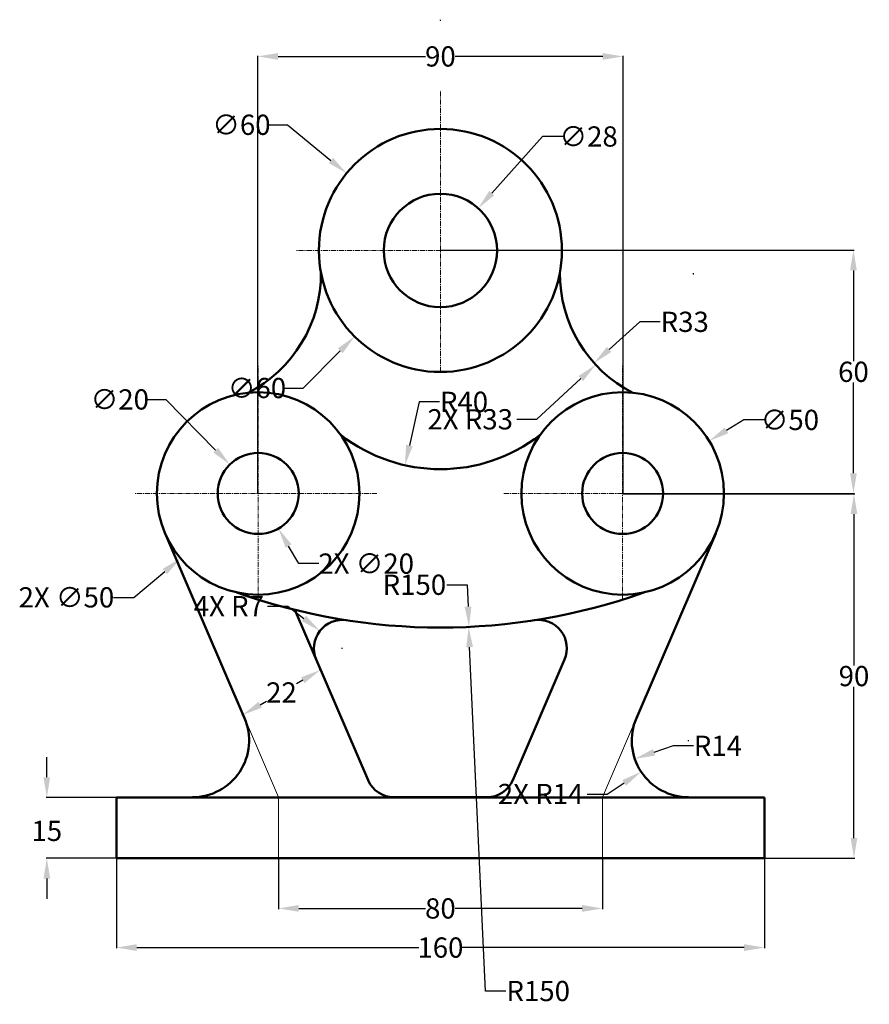
# Model space of a CAD drawing. Units: millimetres. Extents: x 106 to 316, y 45 to 288.
import ezdxf

# ---------------------------------------------------------------- set-up
doc = ezdxf.new("R2010")
doc.units = ezdxf.units.MM
doc.header["$MEASUREMENT"] = 0
doc.linetypes.add('CENTER', pattern=[2, 1.25, -0.25, 0.25, -0.25])
for name, color, linetype, lineweight in [('CENTER', 7, 'CENTER', 18), ('M-CONS', 8, 'Continuous', 13), ('M-DIMS', 2, 'Continuous', 25), ('M-OUTL', 7, 'Continuous', 50)]:
    doc.layers.add(name, color=color, linetype=linetype, lineweight=lineweight)
doc.styles.get("Standard").update_dxf_attribs({"font": 'arial.ttf'})
doc.dimstyles.get("Standard").update_dxf_attribs({"dimtxt": 5, "dimasz": 5, "dimexe": 0.18, "dimexo": 0.0625, "dimgap": 0.09, "dimtad": 0, "dimtih": 1, "dimtoh": 1, "dimdec": 0, "dimzin": 0, "dimdsep": 46, "dimtxsty": 'Standard', "dimcen": 0.09, "dimadec": 0, "dimazin": 0, "dimtfac": 1, "dimtdec": 0, "dimtofl": 0, "dimtmove": 0, "dimatfit": 3, "dimfxl": 1, "dimtolj": 1, "dimtzin": 0, "dimarcsym": 0})

# ---------------------------------------------------------------- blocks, each defined once
blk = doc.blocks.new('*D1')
at = {"layer": 'Defpoints', "color": 0, "transparency": 16777216}
for p in [(210.19, 217.04), (201.44, 178.01)]:
    blk.add_point(p, dxfattribs=at)
at = {"layer": 'M-DIMS', "color": 0, "lineweight": -2, "transparency": 16777216}
for p, q in [((204.95, 193.67), (202.53, 182.89)), ((209.95, 193.67), (204.95, 193.67))]:
    blk.add_line(p, q, dxfattribs=at)
at = {"layer": 'M-DIMS', "color": 0, "transparency": 16777216}
blk.add_solid([(201.72, 183.07), (203.35, 182.7), (201.44, 178.01)], dxfattribs=at)
at = {"layer": 'M-DIMS', "color": 0, "transparency": 16777216, "insert": (216.01, 193.67), "char_height": 5, "attachment_point": 5}
blk.add_mtext('\\A1;R40', dxfattribs=at)
blk = doc.blocks.new('*D2')
at = {"layer": 'Defpoints', "color": 0, "transparency": 16777216}
for p in [(210.19, 287.93), (217.25, 138.1)]:
    blk.add_point(p, dxfattribs=at)
at = {"layer": 'M-DIMS', "color": 0, "lineweight": -2, "transparency": 16777216}
for p, q in [((211.76, 148.5), (216.76, 148.5)), ((216.76, 148.5), (217.01, 143.09))]:
    blk.add_line(p, q, dxfattribs=at)
at = {"layer": 'M-DIMS', "color": 0, "transparency": 16777216}
blk.add_solid([(217.84, 143.13), (216.18, 143.05), (217.25, 138.1)], dxfattribs=at)
at = {"layer": 'M-DIMS', "color": 0, "transparency": 16777216, "insert": (203.76, 148.5), "char_height": 5, "attachment_point": 5}
blk.add_mtext('\\A1;R150', dxfattribs=at)
blk = doc.blocks.new('*D3')
at = {"layer": 'Defpoints', "color": 0, "transparency": 16777216}
for p in [(271.44, 110.04), (258.2, 105.5)]:
    blk.add_point(p, dxfattribs=at)
at = {"layer": 'M-DIMS', "color": 0, "lineweight": -2, "transparency": 16777216}
for p, q in [((267.66, 108.74), (262.93, 107.12)), ((272.66, 108.74), (267.66, 108.74))]:
    blk.add_line(p, q, dxfattribs=at)
at = {"layer": 'M-DIMS', "color": 0, "transparency": 16777216}
blk.add_solid([(262.66, 107.91), (263.2, 106.33), (258.2, 105.5)], dxfattribs=at)
at = {"layer": 'M-DIMS', "color": 0, "transparency": 16777216, "insert": (278.71, 108.74), "char_height": 5, "attachment_point": 5}
blk.add_mtext('\\A1;R14', dxfattribs=at)
blk = doc.blocks.new('*D4')
at = {"layer": 'Defpoints', "color": 0, "transparency": 16777216}
for p in [(272.69, 225.31), (248.14, 203.26)]:
    blk.add_point(p, dxfattribs=at)
at = {"layer": 'M-DIMS', "color": 0, "lineweight": -2, "transparency": 16777216}
for p, q in [((259.45, 213.42), (251.86, 206.6)), ((264.45, 213.42), (259.45, 213.42))]:
    blk.add_line(p, q, dxfattribs=at)
at = {"layer": 'M-DIMS', "color": 0, "transparency": 16777216}
blk.add_solid([(251.3, 207.22), (252.41, 205.98), (248.14, 203.26)], dxfattribs=at)
at = {"layer": 'M-DIMS', "color": 0, "transparency": 16777216, "insert": (270.52, 213.42), "char_height": 5, "attachment_point": 5}
blk.add_mtext('\\A1;R33', dxfattribs=at)
blk = doc.blocks.new('*D5')
at = {"layer": 'Defpoints', "color": 0, "transparency": 16777216}
for p in [(187.02, 250.09), (233.37, 211.99)]:
    blk.add_point(p, dxfattribs=at)
at = {"layer": 'M-DIMS', "color": 0, "lineweight": -2, "transparency": 16777216}
for p, q in [((167.43, 262.07), (172.43, 262.07)), ((172.43, 262.07), (183.15, 253.26)), ((210.1, 231.04), (210.28, 231.04)), ((210.19, 230.95), (210.19, 231.13))]:
    blk.add_line(p, q, dxfattribs=at)
at = {"layer": 'M-DIMS', "color": 0, "transparency": 16777216}
blk.add_solid([(183.68, 253.9), (182.63, 252.62), (187.02, 250.09)], dxfattribs=at)
at = {"layer": 'M-DIMS', "color": 0, "transparency": 16777216, "insert": (161.05, 262.07), "char_height": 5, "attachment_point": 5}
blk.add_mtext('\\A1;∅60', dxfattribs=at)
blk = doc.blocks.new('*D6')
at = {"layer": 'Defpoints', "color": 0, "transparency": 16777216}
for p in [(219.53, 241.47), (200.85, 220.61)]:
    blk.add_point(p, dxfattribs=at)
at = {"layer": 'M-DIMS', "color": 0, "lineweight": -2, "transparency": 16777216}
for p, q in [((235.39, 259.18), (222.87, 245.19)), ((240.39, 259.18), (235.39, 259.18)), ((210.1, 231.04), (210.28, 231.04)), ((210.19, 230.95), (210.19, 231.13))]:
    blk.add_line(p, q, dxfattribs=at)
at = {"layer": 'M-DIMS', "color": 0, "transparency": 16777216}
blk.add_solid([(222.25, 245.75), (223.49, 244.64), (219.53, 241.47)], dxfattribs=at)
at = {"layer": 'M-DIMS', "color": 0, "transparency": 16777216, "insert": (246.79, 259.18), "char_height": 5, "attachment_point": 5}
blk.add_mtext('\\A1;∅28', dxfattribs=at)
blk = doc.blocks.new('*D7')
at = {"layer": 'Defpoints', "color": 0, "transparency": 16777216}
for p in [(276.56, 184.01), (233.82, 158.06)]:
    blk.add_point(p, dxfattribs=at)
at = {"layer": 'M-DIMS', "color": 0, "lineweight": -2, "transparency": 16777216}
for p, q in [((285.11, 189.2), (280.84, 186.61)), ((290.11, 189.2), (285.11, 189.2)), ((255.1, 171.04), (255.28, 171.04)), ((255.19, 170.95), (255.19, 171.13))]:
    blk.add_line(p, q, dxfattribs=at)
at = {"layer": 'M-DIMS', "color": 0, "transparency": 16777216}
blk.add_solid([(280.41, 187.32), (281.27, 185.9), (276.56, 184.01)], dxfattribs=at)
at = {"layer": 'M-DIMS', "color": 0, "transparency": 16777216, "insert": (296.49, 189.2), "char_height": 5, "attachment_point": 5}
blk.add_mtext('\\A1;∅50', dxfattribs=at)
blk = doc.blocks.new('*D8')
at = {"layer": 'Defpoints', "color": 0, "transparency": 16777216}
for p in [(158.19, 178.18), (172.2, 163.9)]:
    blk.add_point(p, dxfattribs=at)
at = {"layer": 'M-DIMS', "color": 0, "lineweight": -2, "transparency": 16777216}
for p, q in [((137.4, 194.26), (142.4, 194.26)), ((142.4, 194.26), (154.69, 181.74)), ((165.1, 171.04), (165.28, 171.04)), ((165.19, 170.95), (165.19, 171.13))]:
    blk.add_line(p, q, dxfattribs=at)
at = {"layer": 'M-DIMS', "color": 0, "transparency": 16777216}
blk.add_solid([(155.28, 182.33), (154.09, 181.16), (158.19, 178.18)], dxfattribs=at)
at = {"layer": 'M-DIMS', "color": 0, "transparency": 16777216, "insert": (131.02, 194.26), "char_height": 5, "attachment_point": 5}
blk.add_mtext('\\A1;∅20', dxfattribs=at)
blk = doc.blocks.new('*D9')
at = {"layer": 'Defpoints', "color": 0, "transparency": 16777216}
for p in [(180.53, 127.44), (181, 126.64), (161.81, 115.56)]:
    blk.add_point(p, dxfattribs=at)
at = {"layer": 'M-DIMS', "color": 0, "lineweight": -2, "transparency": 16777216}
for p, q in [((180.96, 126.69), (180.44, 127.6)), ((176.2, 124.94), (174.63, 124.03)), ((165.68, 118.86), (167.25, 119.77)), ((161.78, 115.62), (161.26, 116.52))]:
    blk.add_line(p, q, dxfattribs=at)
at = {"layer": 'M-DIMS', "color": 0, "transparency": 16777216}
for points in [[(175.79, 125.66), (176.62, 124.22), (180.53, 127.44)], [(165.26, 119.58), (166.09, 118.14), (161.35, 116.36)]]:
    blk.add_solid(points, dxfattribs=at)
at = {"layer": 'M-DIMS', "color": 0, "transparency": 16777216, "insert": (170.94, 121.9), "char_height": 5, "attachment_point": 5}
blk.add_mtext('\\A1;22', dxfattribs=at)
blk = doc.blocks.new('*D10')
at = {"layer": 'Defpoints', "color": 0, "transparency": 16777216}
for p in [(255.28, 278.95), (165.1, 171.04), (255.28, 171.04)]:
    blk.add_point(p, dxfattribs=at)
at = {"layer": 'M-DIMS', "color": 0, "lineweight": -2, "transparency": 16777216}
for p, q in [((165.1, 171.1), (165.1, 279.13)), ((170.1, 278.95), (206.53, 278.95)), ((250.28, 278.95), (213.86, 278.95)), ((255.28, 171.1), (255.28, 279.13))]:
    blk.add_line(p, q, dxfattribs=at)
at = {"layer": 'M-DIMS', "color": 0, "transparency": 16777216}
for points in [[(170.1, 279.78), (170.1, 278.12), (165.1, 278.95)], [(250.28, 279.78), (250.28, 278.12), (255.28, 278.95)]]:
    blk.add_solid(points, dxfattribs=at)
at = {"layer": 'M-DIMS', "color": 0, "transparency": 16777216, "insert": (210.19, 278.95), "char_height": 5, "attachment_point": 5}
blk.add_mtext('\\A1;90', dxfattribs=at)
blk = doc.blocks.new('*D11')
at = {"layer": 'Defpoints', "color": 0, "transparency": 16777216}
for p in [(210.19, 231.13), (255.28, 171.04), (312.18, 171.04)]:
    blk.add_point(p, dxfattribs=at)
at = {"layer": 'M-DIMS', "color": 0, "lineweight": -2, "transparency": 16777216}
for p, q in [((210.26, 231.13), (312.36, 231.13)), ((312.18, 226.13), (312.18, 203.73)), ((312.18, 176.04), (312.18, 198.44)), ((255.35, 171.04), (312.36, 171.04))]:
    blk.add_line(p, q, dxfattribs=at)
at = {"layer": 'M-DIMS', "color": 0, "transparency": 16777216}
for points in [[(311.34, 226.13), (313.01, 226.13), (312.18, 231.13)], [(311.34, 176.04), (313.01, 176.04), (312.18, 171.04)]]:
    blk.add_solid(points, dxfattribs=at)
at = {"layer": 'M-DIMS', "color": 0, "transparency": 16777216, "insert": (312.18, 201.08), "char_height": 5, "attachment_point": 5}
blk.add_mtext('\\A1;60', dxfattribs=at)
blk = doc.blocks.new('*D12')
at = {"layer": 'Defpoints', "color": 0, "transparency": 16777216}
for p in [(255.19, 170.95), (255.19, 80.95), (312.31, 80.95)]:
    blk.add_point(p, dxfattribs=at)
at = {"layer": 'M-DIMS', "color": 0, "lineweight": -2, "transparency": 16777216}
for p, q in [((255.26, 170.95), (312.49, 170.95)), ((312.31, 165.95), (312.31, 128.59)), ((312.31, 85.95), (312.31, 123.31)), ((255.26, 80.95), (312.49, 80.95))]:
    blk.add_line(p, q, dxfattribs=at)
at = {"layer": 'M-DIMS', "color": 0, "transparency": 16777216}
for points in [[(311.48, 165.95), (313.14, 165.95), (312.31, 170.95)], [(311.48, 85.95), (313.14, 85.95), (312.31, 80.95)]]:
    blk.add_solid(points, dxfattribs=at)
at = {"layer": 'M-DIMS', "color": 0, "transparency": 16777216, "insert": (312.31, 125.95), "char_height": 5, "attachment_point": 5}
blk.add_mtext('\\A1;90', dxfattribs=at)
blk = doc.blocks.new('*D13')
at = {"layer": 'Defpoints', "color": 0, "transparency": 16777216}
for p in [(170.19, 80.95), (250.19, 80.95), (250.19, 68.58)]:
    blk.add_point(p, dxfattribs=at)
at = {"layer": 'M-DIMS', "color": 0, "lineweight": -2, "transparency": 16777216}
for p, q in [((170.19, 80.89), (170.19, 68.4)), ((250.19, 80.89), (250.19, 68.4)), ((175.19, 68.58), (206.53, 68.58)), ((245.19, 68.58), (213.86, 68.58))]:
    blk.add_line(p, q, dxfattribs=at)
at = {"layer": 'M-DIMS', "color": 0, "transparency": 16777216}
for points in [[(175.19, 69.42), (175.19, 67.75), (170.19, 68.58)], [(245.19, 69.42), (245.19, 67.75), (250.19, 68.58)]]:
    blk.add_solid(points, dxfattribs=at)
at = {"layer": 'M-DIMS', "color": 0, "transparency": 16777216, "insert": (210.19, 68.58), "char_height": 5, "attachment_point": 5}
blk.add_mtext('\\A1;80', dxfattribs=at)
blk = doc.blocks.new('*D14')
at = {"layer": 'Defpoints', "color": 0, "transparency": 16777216}
for p in [(130.19, 95.95), (113, 80.95), (130.19, 80.95)]:
    blk.add_point(p, dxfattribs=at)
at = {"layer": 'M-DIMS', "color": 0, "lineweight": -2, "transparency": 16777216}
for p, q in [((113, 100.95), (113, 105.95)), ((130.13, 95.95), (112.82, 95.95)), ((130.13, 80.95), (112.82, 80.95)), ((113, 75.95), (113, 70.95))]:
    blk.add_line(p, q, dxfattribs=at)
at = {"layer": 'M-DIMS', "color": 0, "transparency": 16777216}
for points in [[(112.17, 100.95), (113.83, 100.95), (113, 95.95)], [(112.17, 75.95), (113.83, 75.95), (113, 80.95)]]:
    blk.add_solid(points, dxfattribs=at)
at = {"layer": 'M-DIMS', "color": 0, "transparency": 16777216, "insert": (113, 87.73), "char_height": 5, "attachment_point": 5}
blk.add_mtext('\\A1;15', dxfattribs=at)
blk = doc.blocks.new('*D15')
at = {"layer": 'Defpoints', "color": 0, "transparency": 16777216}
for p in [(130.19, 80.95), (290.19, 80.95), (290.19, 58.92)]:
    blk.add_point(p, dxfattribs=at)
at = {"layer": 'M-DIMS', "color": 0, "lineweight": -2, "transparency": 16777216}
for p, q in [((130.19, 80.89), (130.19, 58.74)), ((290.19, 80.89), (290.19, 58.74)), ((135.19, 58.92), (204.82, 58.92)), ((285.19, 58.92), (215.56, 58.92))]:
    blk.add_line(p, q, dxfattribs=at)
at = {"layer": 'M-DIMS', "color": 0, "transparency": 16777216}
for points in [[(135.19, 59.75), (135.19, 58.08), (130.19, 58.92)], [(285.19, 59.75), (285.19, 58.08), (290.19, 58.92)]]:
    blk.add_solid(points, dxfattribs=at)
at = {"layer": 'M-DIMS', "color": 0, "transparency": 16777216, "insert": (210.19, 58.92), "char_height": 5, "attachment_point": 5}
blk.add_mtext('\\A1;160', dxfattribs=at)
blk = doc.blocks.new('BOSS-OD50-BORE20')
for radius in [25, 10]:
    blk.add_circle((25, 25), radius)
blk = doc.blocks.new('*D17')
at = {"layer": 'Defpoints', "color": 0, "transparency": 16777216}
for p in [(231.39, 252.27), (189, 209.81)]:
    blk.add_point(p, dxfattribs=at)
at = {"layer": 'M-DIMS', "color": 0, "lineweight": -2, "transparency": 16777216}
for p, q in [((210.1, 231.04), (210.28, 231.04)), ((210.19, 230.95), (210.19, 231.13)), ((176.28, 197.07), (185.47, 206.27)), ((171.28, 197.07), (176.28, 197.07))]:
    blk.add_line(p, q, dxfattribs=at)
at = {"layer": 'M-DIMS', "color": 0, "transparency": 16777216}
blk.add_solid([(184.88, 206.86), (186.06, 205.68), (189, 209.81)], dxfattribs=at)
at = {"layer": 'M-DIMS', "color": 0, "transparency": 16777216, "insert": (164.9, 197.07), "char_height": 5, "attachment_point": 5}
blk.add_mtext('\\A1;∅60', dxfattribs=at)
blk = doc.blocks.new('*D18')
at = {"layer": 'Defpoints', "color": 0, "transparency": 16777216}
for p in [(184.38, 187.07), (146.01, 155.01)]:
    blk.add_point(p, dxfattribs=at)
at = {"layer": 'M-DIMS', "color": 0, "lineweight": -2, "transparency": 16777216}
for p, q in [((165.1, 171.04), (165.28, 171.04)), ((165.19, 170.95), (165.19, 171.13)), ((134.5, 145.39), (142.17, 151.8)), ((129.5, 145.39), (134.5, 145.39))]:
    blk.add_line(p, q, dxfattribs=at)
at = {"layer": 'M-DIMS', "color": 0, "transparency": 16777216}
blk.add_solid([(141.64, 152.44), (142.71, 151.16), (146.01, 155.01)], dxfattribs=at)
at = {"layer": 'M-DIMS', "color": 0, "transparency": 16777216, "insert": (117.84, 145.39), "char_height": 5, "attachment_point": 5}
blk.add_mtext('\\A1;2X ∅50', dxfattribs=at)
blk = doc.blocks.new('*D19')
at = {"layer": 'Defpoints', "color": 0, "transparency": 16777216}
for p in [(160.19, 179.7), (170.19, 162.38)]:
    blk.add_point(p, dxfattribs=at)
at = {"layer": 'M-DIMS', "color": 0, "lineweight": -2, "transparency": 16777216}
for p, q in [((165.1, 171.04), (165.28, 171.04)), ((165.19, 170.95), (165.19, 171.13)), ((175.2, 153.72), (172.7, 158.05)), ((180.2, 153.72), (175.2, 153.72))]:
    blk.add_line(p, q, dxfattribs=at)
at = {"layer": 'M-DIMS', "color": 0, "transparency": 16777216}
blk.add_solid([(173.42, 158.47), (171.97, 157.63), (170.19, 162.38)], dxfattribs=at)
at = {"layer": 'M-DIMS', "color": 0, "transparency": 16777216, "insert": (191.86, 153.72), "char_height": 5, "attachment_point": 5}
blk.add_mtext('\\A1;2X ∅20', dxfattribs=at)
blk = doc.blocks.new('*D20')
at = {"layer": 'Defpoints', "color": 0, "transparency": 16777216}
for p in [(272.69, 225.31), (248.53, 202.83)]:
    blk.add_point(p, dxfattribs=at)
at = {"layer": 'M-DIMS', "color": 0, "lineweight": -2, "transparency": 16777216}
for p, q in [((272.6, 225.31), (272.78, 225.31)), ((272.69, 225.22), (272.69, 225.4)), ((234.03, 189.35), (244.87, 199.43)), ((229.03, 189.35), (234.03, 189.35))]:
    blk.add_line(p, q, dxfattribs=at)
at = {"layer": 'M-DIMS', "color": 0, "transparency": 16777216}
blk.add_solid([(244.3, 200.04), (245.44, 198.82), (248.53, 202.83)], dxfattribs=at)
at = {"layer": 'M-DIMS', "color": 0, "transparency": 16777216, "insert": (217.55, 189.35), "char_height": 5, "attachment_point": 5}
blk.add_mtext('\\A1;2X R33', dxfattribs=at)
blk = doc.blocks.new('*D21')
at = {"layer": 'Defpoints', "color": 0, "transparency": 16777216}
for p in [(210.19, 287.93), (217.16, 138.09)]:
    blk.add_point(p, dxfattribs=at)
at = {"layer": 'M-DIMS', "color": 0, "lineweight": -2, "transparency": 16777216}
for p, q in [((210.1, 287.93), (210.28, 287.93)), ((210.19, 287.84), (210.19, 288.02)), ((221.34, 48.19), (217.39, 133.1)), ((226.34, 48.19), (221.34, 48.19))]:
    blk.add_line(p, q, dxfattribs=at)
at = {"layer": 'M-DIMS', "color": 0, "transparency": 16777216}
blk.add_solid([(218.23, 133.14), (216.56, 133.06), (217.16, 138.09)], dxfattribs=at)
at = {"layer": 'M-DIMS', "color": 0, "transparency": 16777216, "insert": (234.34, 48.19), "char_height": 5, "attachment_point": 5}
blk.add_mtext('\\A1;R150', dxfattribs=at)
blk = doc.blocks.new('*D22')
at = {"layer": 'Defpoints', "color": 0, "transparency": 16777216}
for p in [(271.44, 110.04), (259.75, 102.34)]:
    blk.add_point(p, dxfattribs=at)
at = {"layer": 'M-DIMS', "color": 0, "lineweight": -2, "transparency": 16777216}
for p, q in [((271.35, 110.04), (271.53, 110.04)), ((271.44, 109.95), (271.44, 110.13)), ((251.4, 96.83), (255.58, 99.59)), ((246.4, 96.83), (251.4, 96.83))]:
    blk.add_line(p, q, dxfattribs=at)
at = {"layer": 'M-DIMS', "color": 0, "transparency": 16777216}
blk.add_solid([(255.12, 100.28), (256.04, 98.89), (259.75, 102.34)], dxfattribs=at)
at = {"layer": 'M-DIMS', "color": 0, "transparency": 16777216, "insert": (234.93, 96.83), "char_height": 5, "attachment_point": 5}
blk.add_mtext('\\A1;2X R14', dxfattribs=at)
blk = doc.blocks.new('*D23')
at = {"layer": 'Defpoints', "color": 0, "transparency": 16777216}
for p in [(180.43, 137.1), (185.96, 132.81)]:
    blk.add_point(p, dxfattribs=at)
at = {"layer": 'M-DIMS', "color": 0, "lineweight": -2, "transparency": 16777216}
for p, q in [((167.53, 143.23), (172.53, 143.23)), ((172.53, 143.23), (176.48, 140.17)), ((185.87, 132.81), (186.05, 132.81)), ((185.96, 132.72), (185.96, 132.9))]:
    blk.add_line(p, q, dxfattribs=at)
at = {"layer": 'M-DIMS', "color": 0, "transparency": 16777216}
blk.add_solid([(177, 140.83), (175.97, 139.51), (180.43, 137.1)], dxfattribs=at)
at = {"layer": 'M-DIMS', "color": 0, "transparency": 16777216, "insert": (157.94, 143.23), "char_height": 5, "attachment_point": 5}
blk.add_mtext('\\A1;4X R7', dxfattribs=at)

msp = doc.modelspace()

# ---------------------------------------------------------------- linework, layer by layer
at = {"layer": 'CENTER'}
for p, q in [((210.19, 201.04), (210.19, 270.56)), ((250.41, 231.04), (174.6, 231.04)), ((165.19, 144.84), (165.19, 202.75)), ((255.19, 144.84), (255.19, 202.75)), ((194.51, 171.04), (134.8, 171.04)), ((225.88, 171.04), (285.58, 171.04))]:
    msp.add_line(p, q, dxfattribs=at)
at = {"layer": 'M-CONS'}
for p, q in [((170.19, 96.04), (157.09, 126.55)), ((250.19, 96.04), (263.3, 126.55)), ((170.19, 80.95), (170.19, 96.04)), ((250.19, 80.95), (250.19, 96.04)), ((250.19, 80.95), (170.19, 80.95))]:
    msp.add_line(p, q, dxfattribs=at)
at = {"layer": 'M-OUTL'}
for p, q in [((161.81, 115.56), (142.22, 161.17)), ((258.58, 115.56), (278.17, 161.17)), ((192.32, 100.28), (174.27, 142.29)), ((228.07, 100.28), (240.86, 130.05)), ((130.19, 80.95), (130.19, 95.95)), ((130.19, 95.95), (290.19, 95.95)), ((198.75, 96.04), (221.64, 96.04)), ((290.19, 95.95), (290.19, 80.95)), ((130.19, 80.95), (290.19, 80.95))]:
    msp.add_line(p, q, dxfattribs=at)
for radius in [30, 14]:
    msp.add_circle((210.19, 231.04), radius, dxfattribs=at)
for centre, radius, start, end in [((147.7, 225.31), 33, 297.0302, 0.4774), ((272.69, 225.31), 33, 179.5226, 242.9698), ((210.19, 217.04), 40, 232.0261, 307.9739), ((210.19, 287.93), 150, 250.4294, 289.5706), ((185.96, 132.81), 7, 81.1219, 203.2404), ((234.42, 132.81), 7, 336.7596, 98.8781), ((148.95, 110.04), 14, 270, 23.2404), ((271.44, 110.04), 14, 156.7596, 270), ((198.75, 103.04), 7, 203.2404, 270), ((221.64, 103.04), 7, 270, 336.7596)]:
    msp.add_arc(centre, radius, start, end, dxfattribs=at)

# ---------------------------------------------------------------- block references
for p in [(140.19, 146.04), (230.19, 146.04)]:
    msp.add_blockref('BOSS-OD50-BORE20', p, dxfattribs=at)

# ---------------------------------------------------------------- dimensions: what is measured, and where the dimension line sits
at = {"layer": 'M-DIMS'}
for center, mpoint, override, picture, middle in [((210.19, 287.93), (217.25, 138.1), {"dimclrd": 0, "dimclre": 0, "dimclrt": 0}, '*D2', (203.76, 148.5)), ((210.19, 287.93), (217.16, 138.09), {"dimdec": 0, "dimlfac": 1, "dimrnd": 0, "dimzin": 0, "dimdsep": 46, "dimlunit": 2}, '*D21', (234.34, 48.19)), ((272.69, 225.31), (248.14, 203.26), {"dimclrd": 0, "dimclre": 0, "dimclrt": 0}, '*D4', (270.52, 213.42)), ((210.19, 217.04), (201.44, 178.01), {"dimclrd": 0, "dimclre": 0, "dimclrt": 0}, '*D1', (216.01, 193.67)), ((271.44, 110.04), (258.2, 105.5), {"dimclrd": 0, "dimclre": 0, "dimclrt": 0}, '*D3', (278.71, 108.74))]:
    dim = msp.add_radius_dim(center=center, mpoint=mpoint, dimstyle='Standard', override=override, dxfattribs=at)
    dim.commit()
    dim.dimension.update_dxf_attribs({"geometry": picture, "text_midpoint": middle, "dimtype": 164})
for base, p1, p2, picture, middle in [((255.28, 278.95), (165.1, 171.04), (255.28, 171.04), '*D10', (210.19, 278.95)), ((290.19, 58.92), (130.19, 80.95), (290.19, 80.95), '*D15', (210.19, 58.92)), ((250.19, 68.58), (170.19, 80.95), (250.19, 80.95), '*D13', (210.19, 68.58))]:
    dim = msp.add_linear_dim(base=base, p1=p1, p2=p2, dimstyle='Standard', override={"dimclrd": 0, "dimclre": 0, "dimclrt": 0}, dxfattribs=at)
    dim.commit()
    dim.dimension.update_dxf_attribs({"geometry": picture, "text_midpoint": middle})
for p1, p2, override, picture, middle in [((233.37, 211.99), (187.02, 250.09), {"dimclrd": 0, "dimclre": 0, "dimclrt": 0}, '*D5', (161.05, 262.07)), ((200.85, 220.61), (219.53, 241.47), {"dimclrd": 0, "dimclre": 0, "dimclrt": 0}, '*D6', (246.79, 259.18)), ((231.39, 252.27), (189, 209.81), {"dimdec": 0, "dimlfac": 1, "dimrnd": 0, "dimzin": 0, "dimdsep": 46, "dimlunit": 2}, '*D17', (164.9, 197.07)), ((172.2, 163.9), (158.19, 178.18), {"dimclrd": 0, "dimclre": 0, "dimclrt": 0}, '*D8', (131.02, 194.26))]:
    dim = msp.add_diameter_dim_2p(p1=p1, p2=p2, dimstyle='Standard', override=override, dxfattribs=at)
    dim.commit()
    dim.dimension.update_dxf_attribs({"geometry": picture, "text_midpoint": middle, "dimtype": 163})
for base, p1, p2, picture, middle in [((312.18, 171.04), (210.19, 231.13), (255.28, 171.04), '*D11', (312.18, 201.08)), ((312.31, 80.95), (255.19, 170.95), (255.19, 80.95), '*D12', (312.31, 125.95))]:
    dim = msp.add_linear_dim(base=base, p1=p1, p2=p2, angle=90, dimstyle='Standard', override={"dimclrd": 0, "dimclre": 0, "dimclrt": 0}, dxfattribs=at)
    dim.commit()
    dim.dimension.update_dxf_attribs({"geometry": picture, "text_midpoint": middle})
dim = msp.add_radius_dim(center=(272.69, 225.31), mpoint=(248.53, 202.83), text='2X <>', dimstyle='Standard', override={"dimdec": 0, "dimlfac": 1, "dimrnd": 0, "dimzin": 0, "dimdsep": 46, "dimlunit": 2}, dxfattribs=at)
dim.commit()
dim.dimension.update_dxf_attribs({"geometry": '*D20', "text_midpoint": (217.55, 189.35), "dimtype": 164})
dim = msp.add_diameter_dim_2p(p1=(233.82, 158.06), p2=(276.56, 184.01), dimstyle='Standard', override={"dimclrd": 0, "dimclre": 0, "dimclrt": 0}, dxfattribs=at)
dim.commit()
dim.dimension.update_dxf_attribs({"geometry": '*D7', "text_midpoint": (296.49, 189.2)})
for p1, p2, picture, middle in [((184.38, 187.07), (146.01, 155.01), '*D18', (117.84, 145.39)), ((160.19, 179.7), (170.19, 162.38), '*D19', (191.86, 153.72))]:
    dim = msp.add_diameter_dim_2p(p1=p1, p2=p2, text='2X <>', dimstyle='Standard', override={"dimdec": 0, "dimlfac": 1, "dimrnd": 0, "dimzin": 0, "dimdsep": 46, "dimlunit": 2}, dxfattribs=at)
    dim.commit()
    dim.dimension.update_dxf_attribs({"geometry": picture, "text_midpoint": middle, "dimtype": 163})
for center, mpoint, text, picture, middle in [((185.96, 132.81), (180.43, 137.1), '4X <>', '*D23', (157.94, 143.23)), ((271.44, 110.04), (259.75, 102.34), '2X <>', '*D22', (234.93, 96.83))]:
    dim = msp.add_radius_dim(center=center, mpoint=mpoint, text=text, dimstyle='Standard', override={"dimdec": 0, "dimlfac": 1, "dimrnd": 0, "dimzin": 0, "dimdsep": 46, "dimlunit": 2}, dxfattribs=at)
    dim.commit()
    dim.dimension.update_dxf_attribs({"geometry": picture, "text_midpoint": middle})
dim = msp.add_aligned_dim(p1=(161.81, 115.56), p2=(181, 126.64), distance=0.92, dimstyle='Standard', override={"dimclrd": 0, "dimclre": 0, "dimclrt": 0}, dxfattribs=at)
dim.commit()
dim.dimension.update_dxf_attribs({"geometry": '*D9', "text_midpoint": (170.94, 121.9)})
dim = msp.add_linear_dim(base=(113, 80.95), p1=(130.19, 95.95), p2=(130.19, 80.95), angle=90, dimstyle='Standard', override={"dimclrd": 0, "dimclre": 0, "dimclrt": 0}, dxfattribs=at)
dim.commit()
dim.dimension.update_dxf_attribs({"geometry": '*D14', "text_midpoint": (113, 87.73), "dimtype": 160})

doc.saveas('drawing.dxf')
